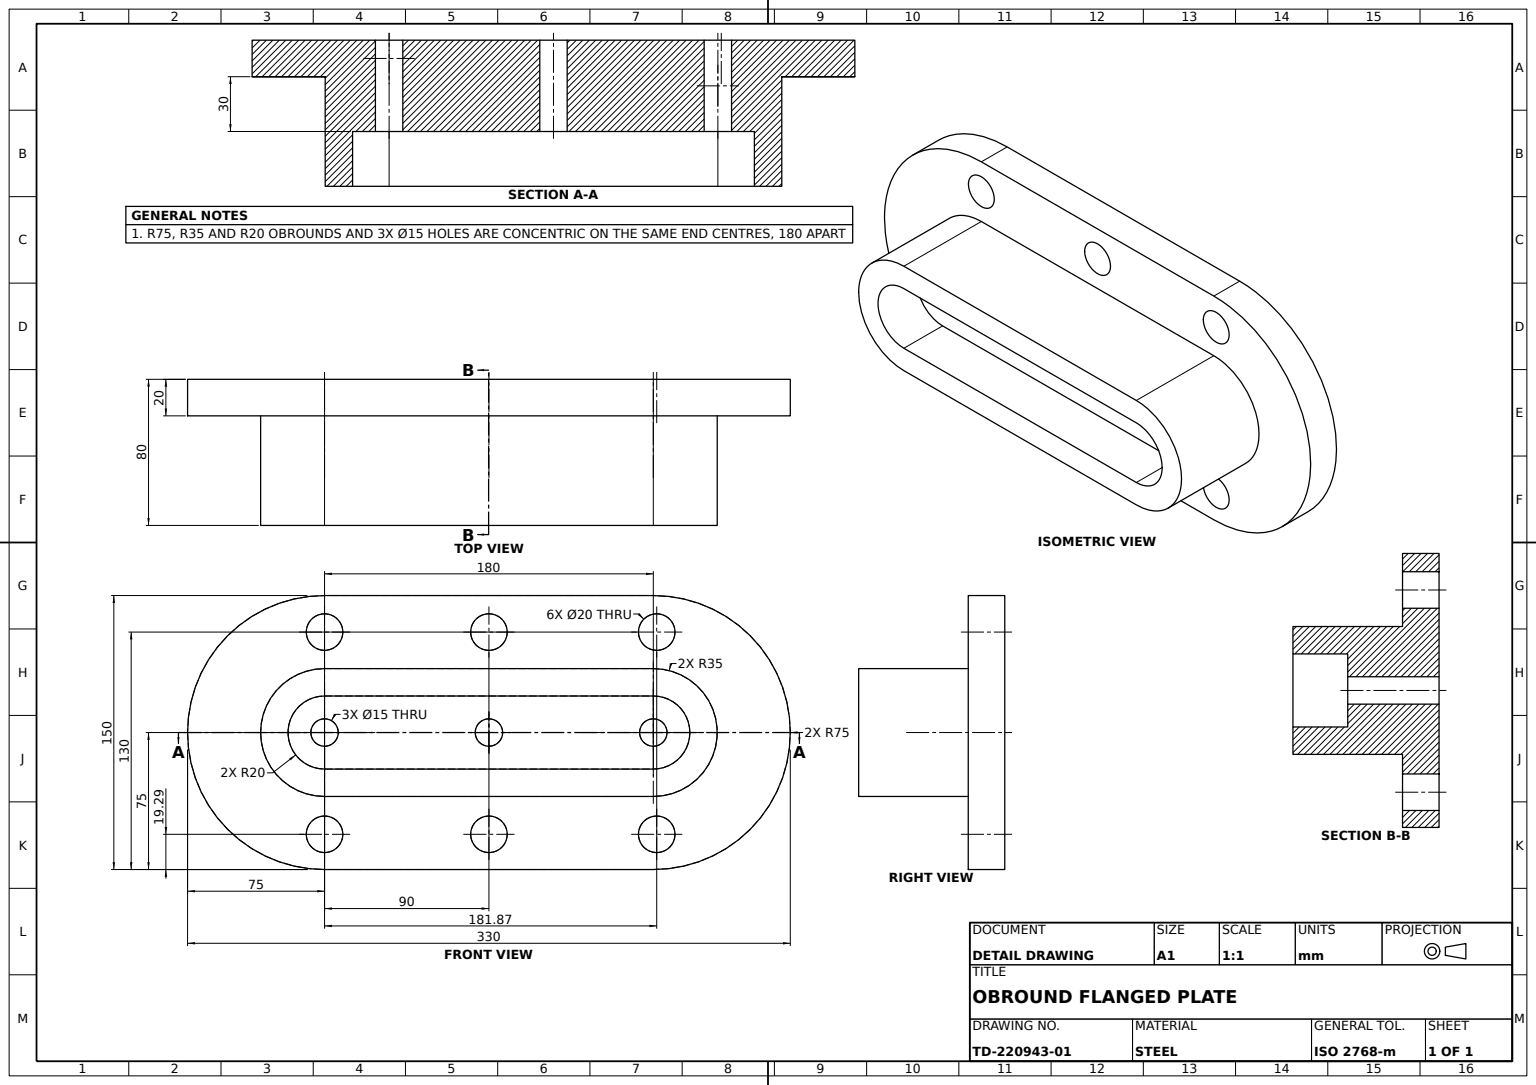
from build123d import *

# Parameters (mm, degrees)
FLANGE_PLATE_DEPTH       = 20
OBROUND_NECK_BOSS_DEPTH  = 60
NECK_POCKET_DEPTH        = 30
THROUGH_OPENING_SKETCH_R = 7.5
THROUGH_OPENING_DEPTH    = 50
MOUNTING_HOLES_SKETCH_R  = 10
MOUNTING_HOLES_DEPTH     = 20


with BuildPart() as part:
    # Flange Plate Sketch → Flange Plate (new body)
    with BuildSketch(Plane.XY):
        with BuildLine():
            Line((0, 75), (180, 75))
            ThreePointArc((180, 75), (255, 0), (180, -75))
            Line((180, -75), (0, -75))
            ThreePointArc((0, -75), (-75, 0), (0, 75))
        make_face()
    extrude(amount=FLANGE_PLATE_DEPTH)

    # Neck Boss Sketch → Obround Neck Boss (add)
    with BuildSketch(Plane.XY.offset(20)):
        with BuildLine():
            Line((0, 35), (180, 35))
            ThreePointArc((180, 35), (215, 0), (180, -35))
            Line((180, -35), (0, -35))
            ThreePointArc((0, -35), (-35, 0), (0, 35))
        make_face()
    extrude(amount=OBROUND_NECK_BOSS_DEPTH)

    # Neck Pocket Sketch → Neck Pocket (cut)
    with BuildSketch(Plane.XY.offset(80)):
        with BuildLine():
            Line((0, 20), (180, 20))
            ThreePointArc((180, 20), (200, 0), (180, -20))
            Line((180, -20), (0, -20))
            ThreePointArc((0, -20), (-20, 0), (0, 20))
        make_face()
    extrude(amount=-NECK_POCKET_DEPTH, mode=Mode.SUBTRACT)

    # Through Opening Sketch → Through Opening (cut)
    with BuildSketch(Plane.XY.offset(50)):
        Circle(THROUGH_OPENING_SKETCH_R)
        with Locations((180, 0)):
            Circle(THROUGH_OPENING_SKETCH_R)
        with Locations((90, 0)):
            Circle(THROUGH_OPENING_SKETCH_R)
    extrude(amount=-THROUGH_OPENING_DEPTH, mode=Mode.SUBTRACT)

    # Mounting Holes Sketch → Mounting Holes (cut)
    with BuildSketch(Plane.XY.offset(20)):
        with Locations((0, 55)):
            Circle(MOUNTING_HOLES_SKETCH_R)
        with Locations((181.871324801, 55)):
            Circle(MOUNTING_HOLES_SKETCH_R)
        with Locations((181.871324801, -55.713132711)):
            Circle(MOUNTING_HOLES_SKETCH_R)
        with Locations((0, -55.713132711)):
            Circle(MOUNTING_HOLES_SKETCH_R)
        with Locations((90, 55)):
            Circle(MOUNTING_HOLES_SKETCH_R)
        with Locations((90, -55.713132711)):
            Circle(MOUNTING_HOLES_SKETCH_R)
    extrude(amount=-MOUNTING_HOLES_DEPTH, mode=Mode.SUBTRACT)


solid = part.part
